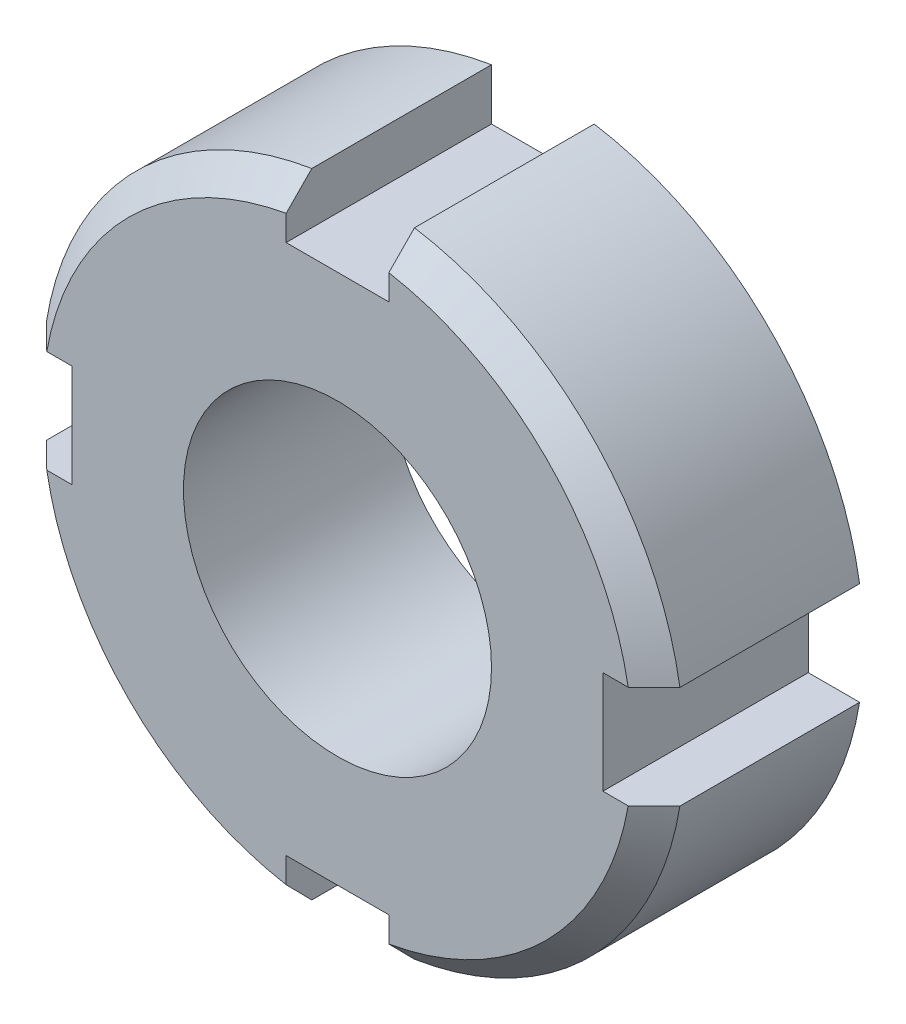
SolidWorks part; units mm, degrees
material "Plain Carbon Steel"
ref_plane "Front Plane" through (0, 0, 0) normal (0, 0, 1) x (1, 0, 0)
ref_plane "Top Plane" through (0, 0, 0) normal (0, 1, 0) x (1, 0, 0)
ref_plane "Right Plane" through (0, 0, 0) normal (1, 0, 0) x (0, 0, -1)
sketch "Slotted Nut Profile" plane through (0, 0, 0) normal (0, 0, 1) x (1, 0, 0)
  line L0 (0, 18.7417) -> (0, -18.1781) construction
  line L1 (-2, 12.339) -> (-2, 10.339)
  line L2 (2, 12.339) -> (2, 10.339)
  line L3 (-2, 10.339) -> (2, 10.339)
  line L4 (12.339, 2) -> (10.339, 2)
  line L5 (-2, 18.7417) -> (-2, -18.1781) construction
  line L6 (2, 18.7417) -> (2, -18.1781) construction
  line L7 (10.339, 2) -> (10.339, -2)
  line L8 (12.339, -2) -> (10.339, -2)
  line L9 (2, -12.339) -> (2, -10.339)
  line L10 (2, -10.339) -> (-2, -10.339)
  line L11 (-2, -12.339) -> (-2, -10.339)
  line L12 (-12.339, -2) -> (-10.339, -2)
  line L13 (-10.339, -2) -> (-10.339, 2)
  line L14 (-12.339, 2) -> (-10.339, 2)
  arc A0 (-2, 12.339) -> (-12.339, 2) centre (0, 0) ccw
  arc A1 (-12.339, -2) -> (-2, -12.339) centre (0, 0) ccw
  arc A2 (2, -12.339) -> (12.339, -2) centre (0, 0) ccw
  arc A3 (12.339, 2) -> (2, 12.339) centre (0, 0) ccw
  point P27 (0, 0)
  dimension "D1" = 25
  dimension "D4" = 2
  dimension "D2" = 2
  dimension "D3" = 2
  dimension "D5" = 4
extrude "Nut Body 8mm" add sketch "Slotted Nut Profile" along normal mid plane 8
hole_wizard "M12 Tapped Hole1" positions "Sketch2" profile "Sketch3" tap size "M12" standard "DIN" end condition through all
sketch "Sketch2" plane through (0, 0, 4) normal (0, 0, 1) x (1, 0, 0)
  point P0 (0, 0)
sketch "Sketch3" plane through (0, 0, 4) normal (1, 0, 0) x (0, -1, 0)
  line L0 (0, 0) -> (0, 8)
  line L1 (0, 8) -> (6, 8)
  line L2 (6, 8) -> (6, 0)
  line L5 (6, 0) -> (0, 0)
  line L11 (0, -6.35) -> (0, 107.95) construction
  dimension "Thru Tap Drill Dia." = 12
  dimension "Thru Tap Drill Depth" = 8
cosmetic thread "Hole Thread1" parameters "D2"=12
chamfer "Edge Chamfer 1x45°" distance 1 angle 45 4 edges at (8.8388, -8.8388, 4) (-8.8388, -8.8388, 4) (-8.8388, 8.8388, 4) (8.8388, 8.8388, 4)
